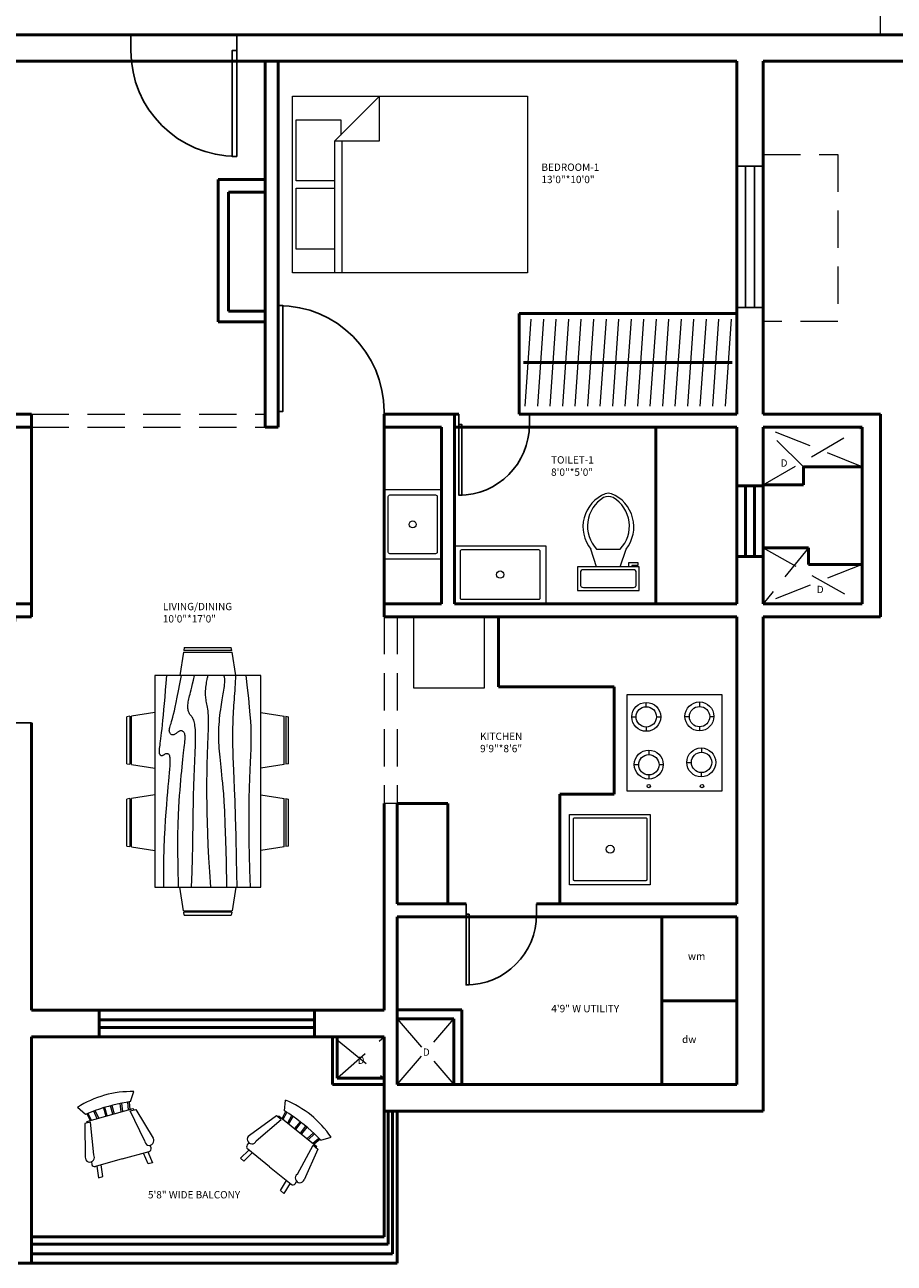
# Model space of a CAD drawing. Units: inches. Extents: x 291 to 2631, y 456 to 2623.
# Tile 5 of 22: x 1167 to 1463, y 513 to 934. Entities that reach past the tile are written whole.
import ezdxf

# ---------------------------------------------------------------- set-up
doc = ezdxf.new("R2010")
doc.units = ezdxf.units.IN
doc.linetypes.add('DASHED', pattern=[19.05, 12.7, -6.35])
for name, color, linetype, lineweight in [('A-ANNO-TEXT', 3, 'Continuous', 25), ('A-AREA-IDEN', 7, 'Continuous', 25), ('A-DOOR', 3, 'Continuous', 25), ('A-EQPM', 8, 'Continuous', 18), ('A-FLOR-FIXT', 9, 'Continuous', 18), ('A-FLOR-OVHD', 1, 'DASHED', 18), ('A-FURN', 8, 'Continuous', 18), ('A-GLAZ', 4, 'Continuous', 25), ('A-WALL', 7, 'Continuous', 50)]:
    doc.layers.add(name, color=color, linetype=linetype, lineweight=lineweight)
doc.styles.get("Standard").update_dxf_attribs({"font": 'arial.ttf'})

# ---------------------------------------------------------------- blocks, each defined once
blk = doc.blocks.new('*U2')
for p, q in [((0, 0), (0, -6)), ((40, 0), (40, -6))]:
    blk.add_line(p, q)
blk.add_lwpolyline([(0, 0), (0, 40), (1.75, 40), (1.75, 0)], close=True)
blk.add_arc((0, 0), 40, 0, 90)
blk = doc.blocks.new('Toilet - top')
for p, q in [((9.5, -6), (9.5, -2)), ((-8, -8.5), (-8, -8)), ((-7, -8), (-7, -9.5)), ((-4, -8), (-6, -14)), ((4, -8), (6, -14)), ((-10, -8.5), (-8, -8.5)), ((-10, -9.5), (-10, -8.5)), ((-7, -9.5), (-10, -9.5)), ((4, -14), (-4, -14))]:
    blk.add_line(p, q)
blk.add_lwpolyline([(10.5, -8), (10.5, 0), (-10.5, 0), (-10.5, -8)], close=True)
for points in [[(-9.5, -2), (-9.5, -6)], [(8.5, -1), (-8.5, -1)], [(-8.5, -7), (8.5, -7)]]:
    blk.add_lwpolyline(points)
for centre, radius, start, end in [((-8.62, -1.88), 0.884, 81.8699, 188.1301), ((8.62, -1.88), 0.884, 351.8699, 98.1301), ((-8.62, -6.12), 0.884, 171.8699, 278.1301), ((8.62, -6.12), 0.884, 261.8699, 8.1301), ((3.52, -21.58), 12.17, 141.4691, 247.9714), ((4.2, -21.82), 11.33, 136.3677, 238.9468), ((-3.52, -21.58), 12.17, 292.0284, 38.5307), ((-4.2, -21.82), 11.33, 301.053, 43.6321), ((0, -27.88), 4, 245.7318, 294.2682), ((0, -29), 4, 254.8605, 285.1395)]:
    blk.add_arc(centre, radius, start, end)
blk = doc.blocks.new('Dining Set - 36 x 72 in.')
for p, q in [((-22.2343, 26.00059), (-23.4847, 17.99762)), ((-22.2304, 26), (-5.7608, 26)), ((-22, 27.5), (-22.1562, 26.50042)), ((-5.8416, 26.5), (-22.1534, 26.5)), ((-22, 27.5), (-6, 27.5)), ((-5.8437, 26.49966), (-6, 27.5)), ((-4.5152, 17.99762), (-5.7655, 25.99926)), ((5.7657, 26.00059), (4.5153, 17.99762)), ((5.7696, 26), (22.2392, 26)), ((6, 27.5), (5.8438, 26.50042)), ((22.1584, 26.5), (5.8466, 26.5)), ((6, 27.5), (22, 27.5)), ((22.1563, 26.49966), (22, 27.5)), ((23.4848, 17.99762), (22.2345, 25.99926)), ((36, 18), (-36, 18)), ((-36, 18), (-36, -18)), ((36, -18), (36, 18)), ((-44.0006, 8.23428), (-35.9976, 9.48474)), ((44.0006, 8.23428), (35.9976, 9.48474)), ((-45.5, 8), (-44.5004, 8.15617)), ((-45.5, 8), (-45.5, -8)), ((-44.5, -8.15843), (-44.5, 8.15338)), ((-44, 8.23041), (-44, -8.23915)), ((44, 8.23041), (44, -8.23915)), ((44.5, -8.15843), (44.5, 8.15338)), ((45.5, 8), (44.5005, 8.15617)), ((45.5, 8), (45.5, -8)), ((-44.4997, -8.15631), (-45.5, -8)), ((-35.9976, -9.48476), (-43.9993, -8.2345)), ((35.9976, -9.48476), (43.9993, -8.2345)), ((44.4997, -8.15631), (45.5, -8)), ((-36, -18), (36, -18)), ((-22.2343, -26.0006), (-23.4847, -17.99762)), ((-4.5152, -17.99762), (-5.7655, -25.99928)), ((5.7657, -26.0006), (4.5153, -17.99762)), ((23.4848, -17.99762), (22.2345, -25.99928)), ((-22.2304, -26), (-5.7608, -26)), ((-22, -27.5), (-22.1562, -26.50044)), ((-5.8416, -26.5), (-22.1534, -26.5)), ((-22, -27.5), (-6, -27.5)), ((-5.8437, -26.49967), (-6, -27.5)), ((5.7696, -26), (22.2392, -26)), ((6, -27.5), (5.8438, -26.50044)), ((22.1584, -26.5), (5.8466, -26.5)), ((6, -27.5), (22, -27.5)), ((22.1563, -26.49967), (22, -27.5))]:
    blk.add_line(p, q)
for points in [[(-36, 15), (-31.1772, 14.97754), (-26.8079, 14.91406), (-22.8538, 14.81543), (-19.276, 14.6875), (-16.0362, 14.53613), (-13.0957, 14.36718), (-10.4159, 14.18652), (-7.9583, 14), (-5.6904, 13.81315), (-3.6035, 13.63021), (-1.6954, 13.45508), (0.0365, 13.29166), (1.5945, 13.14388), (2.9811, 13.01562), (4.1988, 12.9108), (5.25, 12.83333), (6.1393, 12.78613), (6.8802, 12.76823), (7.4883, 12.77767), (7.9792, 12.8125), (8.3685, 12.87077), (8.6719, 12.95052), (8.9049, 13.0498), (9.0833, 13.16666), (9.2205, 13.29899), (9.3216, 13.44401), (9.3895, 13.59879), (9.4271, 13.76041), (9.4373, 13.92594), (9.4232, 14.09245), (9.3875, 14.257), (9.3333, 14.41666), (9.2638, 14.56917), (9.1836, 14.71484), (9.0975, 14.85465), (9.0104, 14.98958), (8.9272, 15.1206), (8.8529, 15.2487), (8.7922, 15.37483), (8.75, 15.5), (8.7305, 15.62467), (8.7344, 15.74739), (8.7617, 15.86621), (8.8125, 15.97916), (8.8867, 16.08431), (8.9844, 16.17968), (9.1055, 16.26334), (9.25, 16.33333), (9.4189, 16.38802), (9.6172, 16.42708), (9.8506, 16.45052), (10.125, 16.45833), (10.4463, 16.45052), (10.8203, 16.42708), (11.2529, 16.38802), (11.75, 16.33333), (12.3184, 16.26318), (12.9694, 16.17838), (13.7151, 16.07991), (14.5677, 15.96875), (15.5395, 15.84586), (16.6426, 15.71224), (17.8893, 15.56884), (19.2917, 15.41666), (20.859, 15.25667), (22.5879, 15.08984), (24.4721, 14.91715), (26.5052, 14.73958), (28.6809, 14.5581), (30.9929, 14.3737), (33.4347, 14.18733), (36, 14)], [(-36, 10), (-28.9766, 10.14274), (-23.1725, 10.20442), (-18.4241, 10.19775), (-14.5677, 10.13541), (-11.4399, 10.03011), (-8.877, 9.89453), (-6.7154, 9.74137), (-4.7917, 9.58333), (-2.9698, 9.43082), (-1.2246, 9.28515), (0.4415, 9.14534), (2.026, 9.01041), (3.5266, 8.87939), (4.9408, 8.7513), (6.266, 8.62516), (7.5, 8.5), (8.6411, 8.37549), (9.6914, 8.2539), (10.6538, 8.13818), (11.5312, 8.03125), (12.3267, 7.93603), (13.043, 7.85547), (13.6831, 7.79248), (14.25, 7.75), (14.7471, 7.7303), (15.1797, 7.73307), (15.5537, 7.75732), (15.875, 7.80208), (16.1494, 7.86637), (16.3828, 7.94922), (16.5811, 8.04964), (16.75, 8.16666), (16.8944, 8.29915), (17.0143, 8.44531), (17.1089, 8.60319), (17.1771, 8.77083), (17.218, 8.94629), (17.2305, 9.1276), (17.2137, 9.31282), (17.1667, 9.5), (17.0895, 9.6875), (16.987, 9.875), (16.8649, 10.0625), (16.7292, 10.25), (16.5856, 10.4375), (16.4401, 10.625), (16.2985, 10.8125), (16.1667, 11), (16.05, 11.18733), (15.9518, 11.3737), (15.8752, 11.5581), (15.8229, 11.73958), (15.798, 11.91715), (15.8034, 12.08984), (15.842, 12.25667), (15.9167, 12.41666), (16.0295, 12.56836), (16.1784, 12.70833), (16.3605, 12.83268), (16.5729, 12.9375), (16.8127, 13.01888), (17.0768, 13.07291), (17.3625, 13.0957), (17.6667, 13.08333), (17.9894, 13.03312), (18.3418, 12.94726), (18.7382, 12.82918), (19.1927, 12.68229), (19.7195, 12.51001), (20.3327, 12.31575), (21.0465, 12.10294), (21.875, 11.875), (22.8357, 11.63354), (23.959, 11.37304), (25.2786, 11.08618), (26.8282, 10.76562), (28.6414, 10.40405), (30.752, 9.99414), (33.1936, 9.52856), (36, 9)], [(-36, 5.5), (-30.7157, 5.3348), (-26.069, 5.20963), (-21.9946, 5.11767), (-18.4271, 5.05208), (-15.3009, 5.00602), (-12.5508, 4.97265), (-10.1112, 4.94515), (-7.9167, 4.91666), (-5.909, 4.88167), (-4.0586, 4.83984), (-2.3429, 4.79215), (-0.7396, 4.73958), (0.7739, 4.6831), (2.22, 4.6237), (3.6213, 4.56233), (5, 4.5), (6.373, 4.43782), (7.7344, 4.3776), (9.0723, 4.32129), (10.375, 4.27083), (11.6309, 4.22819), (12.8281, 4.19531), (13.9551, 4.17415), (15, 4.16666), (15.954, 4.17448), (16.819, 4.19791), (17.6001, 4.23698), (18.3021, 4.29166), (18.9299, 4.36198), (19.4883, 4.44791), (19.9823, 4.54948), (20.4167, 4.66666), (20.7969, 4.79899), (21.1302, 4.94401), (21.4245, 5.09879), (21.6875, 5.26041), (21.9271, 5.42594), (22.1511, 5.59245), (22.3672, 5.757), (22.5834, 5.91666), (22.8065, 6.06868), (23.0404, 6.21093), (23.2879, 6.34147), (23.5521, 6.45833), (23.8358, 6.55957), (24.142, 6.64323), (24.4735, 6.70735), (24.8334, 6.75), (25.2235, 6.76969), (25.642, 6.76692), (26.0858, 6.74267), (26.5521, 6.69791), (27.0379, 6.63362), (27.5404, 6.55078), (28.0565, 6.45036), (28.5834, 6.33333), (29.1242, 6.19987), (29.7071, 6.04687), (30.3661, 5.87044), (31.1354, 5.66666), (32.0493, 5.43164), (33.142, 5.16146), (34.4475, 4.85221), (36, 4.5)], [(-36, -1), (-30.7915, -0.6591), (-26.0195, -0.38216), (-21.6519, -0.16284), (-17.6563, 0.00521), (-14.0005, 0.12833), (-10.6523, 0.21289), (-7.5796, 0.26522), (-4.75, 0.29166), (-2.134, 0.29793), (0.2878, 0.28711), (2.5317, 0.26163), (4.6146, 0.22396), (6.5529, 0.17651), (8.3633, 0.12174), (10.0623, 0.06209), (11.6667, 0), (13.1899, -0.06201), (14.6341, -0.1211), (15.9982, -0.17432), (17.2813, -0.21875), (18.4823, -0.25147), (19.6003, -0.26953), (20.6343, -0.27002), (21.5834, -0.25), (22.4481, -0.20768), (23.2357, -0.14584), (23.9549, -0.06836), (24.6146, 0.02083), (25.2235, 0.11784), (25.7904, 0.21875), (26.3241, 0.31966), (26.8334, 0.41666), (27.3265, 0.50618), (27.8099, 0.58593), (28.2894, 0.65397), (28.7709, 0.70833), (29.2601, 0.74707), (29.763, 0.76823), (30.2855, 0.76985), (30.8334, 0.75), (31.4088, 0.70784), (31.9994, 0.64713), (32.589, 0.57275), (33.1615, 0.48958), (33.7008, 0.4025), (34.1908, 0.3164), (34.6153, 0.23616), (34.9584, 0.16666), (35.2099, 0.11165), (35.3848, 0.07031), (35.504, 0.04069), (35.5886, 0.02083), (35.6594, 0.00879), (35.7377, 0.0026), (35.8442, 0.00032), (36, 0)], [(-36, -6.5), (-27.1843, -6.31267), (-20.084, -6.1263), (-14.469, -5.9419), (-10.1094, -5.76042), (-6.7752, -5.58285), (-4.2363, -5.41016), (-2.2629, -5.24333), (-0.625, -5.08334), (0.8708, -4.93099), (2.2715, -4.78646), (3.5872, -4.64974), (4.8281, -4.52084), (6.0046, -4.39974), (7.127, -4.28646), (8.2053, -4.18099), (9.25, -4.08334), (10.2705, -3.99382), (11.2734, -3.91407), (12.2647, -3.84603), (13.25, -3.79167), (14.2354, -3.75293), (15.2266, -3.73177), (16.2295, -3.73015), (17.25, -3.75), (18.2912, -3.79248), (19.3451, -3.85547), (20.4009, -3.93604), (21.4479, -4.03125), (22.4754, -4.13819), (23.4727, -4.25391), (24.4289, -4.37549), (25.3334, -4.5), (26.1785, -4.62492), (26.9694, -4.74935), (27.7145, -4.87281), (28.4219, -4.99479), (29.1, -5.11483), (29.7572, -5.23242), (30.4016, -5.34709), (31.0417, -5.45834), (31.6837, -5.56437), (32.3262, -5.65821), (32.9658, -5.73153), (33.599, -5.77604), (34.2224, -5.78345), (34.8327, -5.74545), (35.4264, -5.65373), (36, -5.5)], [(-36, -10), (-26.4022, -9.81299), (-18.4675, -9.62891), (-11.9839, -9.45069), (-6.7396, -9.28125), (-2.5226, -9.12354), (0.8789, -8.98047), (3.6769, -8.85498), (6.0833, -8.75), (8.2767, -8.66765), (10.3021, -8.60677), (12.1712, -8.56543), (13.8958, -8.54167), (15.4876, -8.53353), (16.9583, -8.53907), (18.3197, -8.55632), (19.5834, -8.58334), (20.7616, -8.61841), (21.8685, -8.66081), (22.9188, -8.71004), (23.9271, -8.76563), (24.9081, -8.82707), (25.8763, -8.89388), (26.8465, -8.96558), (27.8334, -9.04167), (28.8474, -9.12118), (29.8828, -9.20117), (30.93, -9.27824), (31.9792, -9.34896), (33.0205, -9.40991), (34.0443, -9.45768), (35.0407, -9.48885), (36, -9.5)], [(-36, -14.5), (-30.0881, -14.33513), (-25.0332, -14.21224), (-20.7312, -14.12647), (-17.0781, -14.07292), (-13.97, -14.04671), (-11.3027, -14.04297), (-8.9724, -14.05681), (-6.875, -14.08334), (-4.9224, -14.11833), (-3.0905, -14.16016), (-1.3709, -14.20785), (0.2448, -14.26042), (1.7647, -14.3169), (3.1973, -14.3763), (4.5507, -14.43767), (5.8333, -14.5), (7.0554, -14.5621), (8.235, -14.62175), (9.3922, -14.67652), (10.5469, -14.72396), (11.7192, -14.76164), (12.929, -14.78711), (14.1965, -14.79794), (15.5417, -14.79167), (16.9933, -14.76424), (18.6152, -14.70508), (20.4804, -14.60197), (22.6615, -14.44271), (25.2312, -14.21509), (28.2624, -13.9069), (31.8277, -13.50594), (36, -13)]]:
    blk.add_lwpolyline(points)
blk = doc.blocks.new('Chair - Rocking')
for p, q in [((-8, -4.5), (-10, -1.5)), ((-4.5, -7), (-4.96674, -4.19951)), ((-4, -7), (-4.40532, -4.16272)), ((-1.5, -4.05012), (-1.5, -7)), ((-1, -7), (-1, -4.05012)), ((1, -7), (1, -4.04655)), ((1.5, -4.05012), (1.5, -7)), ((4, -7), (4.40187, -4.18694)), ((4.5, -7), (4.96761, -4.19437)), ((8, -4.5), (10, -1.5)), ((-9, -7.5), (-12, -18.49999)), ((-7, -7.5), (-9, -7.5)), ((-9, -18.49999), (-7, -7.5)), ((-8.23428, -6.99939), (-8.3093, -7.47958)), ((-8.23041, -7), (8.23915, -7)), ((-7.5, -4.5), (-7, -7)), ((-6.5, -7), (-7.02225, -4.43)), ((6.5, -7), (7, -4.4057)), ((7.5, -4.5), (7, -7)), ((7, -7.5), (9, -7.5)), ((9, -18.49999), (7, -7.5)), ((8.31071, -7.48854), (8.23449, -7.00073)), ((9, -7.5), (12, -18.49999)), ((-10.36644, -20.64523), (-10.5, -21.49999)), ((10.5, -21.49999), (10.3575, -20.58798)), ((-9, -22.49999), (-9.5, -26.49999)), ((0, -22.49999), (-9.5, -22.49999)), ((-8, -26.49999), (-7.5, -22.49999)), ((0, -22.49999), (9.5, -22.49999)), ((8, -26.49999), (7.5, -22.49999)), ((9, -22.49999), (9.5, -26.49999)), ((-9.5, -26.49999), (-8, -26.49999)), ((9.5, -26.49999), (8, -26.49999))]:
    blk.add_line(p, q)
for centre, radius, start, end in [((0, -34.08333), 34.08333, 72.93847, 107.0615), ((0, -68.25004), 64.25, 93.92211, 97.15267), ((0, -68.25004), 64.25, 82.84733, 93.92211), ((-10.5, -18.99999), 1.58114, 161.5651, 18.43495), ((10.5, -18.99999), 1.58114, 161.5651, 18.43495), ((-9.5, -21.49999), 1, 180, 270), ((9.5, -21.49999), 1, 270, 0)]:
    blk.add_arc(centre, radius, start, end)
blk = doc.blocks.new('Bed - Queen')
for p, q in [((0, -80.00003), (0, 0)), ((0, 0), (59.99999, 0)), ((59.99999, 0), (59.99999, -80.00003)), ((7.99999, -1.2), (28.79998, -1.2)), ((7.99999, -14.4), (7.99999, -1.2)), ((28.79998, -1.2), (28.79998, -14.4)), ((31.19999, -1.2), (51.99999, -1.2)), ((31.19999, -14.4), (31.19999, -1.2)), ((51.99999, -1.2), (51.99999, -16.4)), ((0, -14.4), (44.8, -14.4)), ((44.8, -16.8), (0, -16.8)), ((59.99999, -29.6), (44.8, -14.4)), ((44.8, -14.4), (44.8, -29.6)), ((51.99999, -16.4), (46.79936, -16.4)), ((44.8, -29.6), (59.99999, -29.6)), ((59.99999, -80.00003), (0, -80.00003))]:
    blk.add_line(p, q)
blk = doc.blocks.new('WIN-1200')
for p, q in [((0, 0), (0, 48)), ((0, 48), (9, 48)), ((3, 0), (3, 48)), ((6, 48), (6, 0)), ((9, 48), (9, 0)), ((9, 0), (0, 0))]:
    blk.add_line(p, q)
blk = doc.blocks.new('COOKTOP-B')
for p, q in [((6.54, 28.68), (6.54, 30.14)), ((24.62, 30.31), (24.62, 28.76)), ((19.7, 25.39), (21.21, 25.39)), ((28.13, 25.39), (29.54, 25.39)), ((1.62, 25.22), (3.08, 25.22)), ((6.54, 21.76), (6.54, 20.3)), ((10, 25.22), (11.46, 25.22)), ((24.62, 21.83), (24.62, 20.47)), ((7.38, 13.92), (7.38, 12.38)), ((25.35, 14.65), (25.34, 13.21)), ((2.46, 9), (3.95, 9)), ((10.87, 9), (12.3, 9)), ((20.32, 9.73), (21.89, 9.73)), ((7.38, 5.46), (7.38, 4.08)), ((25.26, 6.28), (25.24, 4.81))]:
    blk.add_line(p, q)
blk.add_lwpolyline([(0, 32.79), (32.25, 32.79), (32.25, 0), (0, 0)], close=True)
for centre, radius in [((6.54, 25.22), 4.92), ((24.62, 25.39), 4.92), ((6.54, 25.22), 3.46), ((24.67, 25.29), 3.46), ((7.38, 9), 4.92), ((25.24, 9.73), 4.92), ((25.35, 9.74), 3.46), ((7.41, 8.92), 3.46), ((7.38, 1.69), 0.572), ((25.5, 1.69), 0.572)]:
    blk.add_circle(centre, radius)

msp = doc.modelspace()

# ---------------------------------------------------------------- linework, layer by layer
at = {"layer": 'A-FLOR-OVHD'}
for p, q in [((1458.34, 1111.65), (1458.34, 930.98)), ((1418.5, 890.21), (1443.93, 890.21)), ((1443.93, 890.21), (1443.93, 833.45)), ((1443.93, 833.45), (1418.5, 833.45)), ((1169.5, 801.98), (1249, 801.98)), ((1169.5, 797.48), (1249, 797.48)), ((1452.18, 784.08), (1418.5, 797.48)), ((1418.5, 777.9), (1452.18, 797.48)), ((1432.19, 784.08), (1418.5, 797.48)), ((1418.5, 756.5), (1452.18, 737.48)), ((1433.89, 756.5), (1418.5, 737.48)), ((1452.18, 750.84), (1418.5, 737.48)), ((1289.5, 732.98), (1289.5, 669.54)), ((1294, 732.98), (1294, 669.54)), ((1294, 669.54), (1289.5, 669.54)), ((1294, 596.39), (1313.26, 573.98)), ((1294, 573.98), (1313.26, 596.39)), ((1273.6, 590.24), (1273.6, 589.22)), ((1273.6, 576.12), (1289.5, 590.24)), ((1273.6, 589.22), (1289.5, 576.12))]:
    msp.add_line(p, q, dxfattribs=at)
at = {"layer": 'A-FURN'}
for p, q in [((1337.54, 804.7), (1339.61, 834.23)), ((1341.8, 804.7), (1343.86, 834.23)), ((1346.05, 804.7), (1348.12, 834.23)), ((1350.31, 804.7), (1352.37, 834.23)), ((1354.56, 804.7), (1356.63, 834.23)), ((1358.82, 804.7), (1360.88, 834.23)), ((1363.07, 804.7), (1365.14, 834.23)), ((1367.33, 804.7), (1369.4, 834.23)), ((1371.59, 804.7), (1373.65, 834.23)), ((1375.84, 804.7), (1377.91, 834.23)), ((1380.1, 804.7), (1382.16, 834.23)), ((1384.35, 804.7), (1386.42, 834.23)), ((1388.61, 804.7), (1390.68, 834.23)), ((1392.86, 804.7), (1394.93, 834.23)), ((1397.12, 804.7), (1399.19, 834.23)), ((1401.38, 804.7), (1403.44, 834.23)), ((1405.63, 804.7), (1407.7, 834.23))]:
    msp.add_line(p, q, dxfattribs=at)
for points in [[(1289.5, 776.29), (1309, 776.29), (1309, 752.63), (1289.5, 752.63)], [(1313.5, 737.48), (1344.66, 737.48), (1344.66, 757.06), (1313.5, 757.06)], [(1299.65, 732.98), (1323.58, 732.98), (1323.58, 708.81), (1299.65, 708.81)], [(1352.65, 665.8), (1380.09, 665.8), (1380.09, 641.9), (1352.65, 641.9)]]:
    msp.add_lwpolyline(points, close=True, dxfattribs=at)
for points in [[(1291.46, 774.47), (1307.06, 774.47, -0.414214), (1307.56, 773.97), (1307.56, 755, -0.414214), (1307.06, 754.5), (1291.46, 754.5, -0.414214), (1290.96, 755), (1290.96, 773.97, -0.414214)], [(1315.87, 739), (1342.16, 739, 0.414214), (1342.66, 739.5), (1342.66, 755.27, 0.414214), (1342.16, 755.77), (1315.87, 755.77, 0.414214), (1315.37, 755.27), (1315.37, 739.5, 0.414214)], [(1354.29, 664.69), (1378.59, 664.69, -0.414214), (1378.89, 664.39), (1378.89, 643.61, -0.414214), (1378.59, 643.31), (1354.29, 643.31, -0.414214), (1353.99, 643.61), (1353.99, 664.39, -0.414214)]]:
    msp.add_lwpolyline(points, format="xyb", close=True, dxfattribs=at)
for centre, radius in [((1299.26, 764.48), 1.16), ((1329.01, 747.38), 1.24), ((1366.44, 654), 1.36)]:
    msp.add_circle(centre, radius, dxfattribs=at)
at = {"layer": 'A-WALL'}
for p, q in [((1989.87, 930.98), (1024, 930.98)), ((1409.5, 921.98), (1033, 921.98)), ((1249, 921.98), (1249, 797.48)), ((1253.5, 921.98), (1253.5, 797.48)), ((1409.5, 921.98), (1409.5, 801.98)), ((1595.37, 921.98), (1418.5, 921.98)), ((1418.5, 921.98), (1418.5, 801.98)), ((1249, 881.72), (1233.03, 881.72)), ((1233.03, 881.72), (1233.03, 833.39)), ((1249, 877.47), (1236.59, 877.47)), ((1236.59, 877.47), (1236.59, 836.95)), ((1236.59, 836.95), (1249, 836.95)), ((1335.52, 801.98), (1335.52, 836.12)), ((1335.52, 836.12), (1409.5, 836.12)), ((1233.03, 833.39), (1249, 833.39)), ((1336.9, 819.47), (1407.94, 819.47)), ((1169.5, 801.98), (1033, 801.98)), ((1169.5, 737.48), (1169.5, 801.98)), ((1289.5, 737.48), (1289.5, 801.98)), ((1314.97, 801.98), (1289.5, 801.98)), ((1313.5, 801.98), (1313.5, 737.48)), ((1409.5, 801.98), (1335.52, 801.98)), ((1418.5, 801.98), (1458.38, 801.98)), ((1458.38, 801.98), (1458.38, 732.98)), ((1169.5, 797.48), (1145.5, 797.48)), ((1253.5, 797.48), (1249, 797.48)), ((1309, 797.48), (1289.5, 797.48)), ((1309, 797.48), (1309, 737.48)), ((1409.5, 797.48), (1313.5, 797.48)), ((1381.97, 797.48), (1381.97, 737.48)), ((1409.5, 797.48), (1409.5, 737.48)), ((1418.5, 797.48), (1452.18, 797.48)), ((1418.5, 797.48), (1418.5, 737.48)), ((1452.18, 797.48), (1452.18, 737.48)), ((1432.19, 777.9), (1432.19, 784.08)), ((1432.19, 784.08), (1452.18, 784.08)), ((1418.5, 777.55), (1409.5, 777.55)), ((1409.5, 777.55), (1409.5, 753.55)), ((1412.5, 777.55), (1412.5, 753.55)), ((1415.5, 753.55), (1415.5, 777.55)), ((1418.5, 777.9), (1432.19, 777.9)), ((1418.5, 753.55), (1418.5, 777.55)), ((1418.5, 756.5), (1433.89, 756.5)), ((1433.89, 756.5), (1433.89, 750.84)), ((1409.5, 753.55), (1418.5, 753.55)), ((1433.89, 750.84), (1452.18, 750.84)), ((1169.5, 737.48), (1145.5, 737.48)), ((1169.5, 737.48), (1169.5, 732.98)), ((1289.5, 737.48), (1289.5, 732.98)), ((1309, 737.48), (1289.5, 737.48)), ((1409.5, 737.48), (1313.5, 737.48)), ((1452.18, 737.48), (1418.5, 737.48)), ((1169.5, 732.98), (1105.76, 732.98)), ((1409.5, 732.98), (1289.5, 732.98)), ((1328.43, 709.22), (1328.43, 732.98)), ((1409.5, 732.98), (1409.5, 635.48)), ((1458.38, 732.98), (1418.5, 732.98)), ((1418.5, 732.98), (1418.5, 564.98)), ((1367.84, 709.22), (1328.43, 709.22)), ((1367.84, 672.71), (1367.84, 709.22)), ((1169.5, 696.98), (1169.5, 599.24)), ((1349.26, 635.48), (1349.26, 672.71)), ((1349.26, 672.71), (1367.84, 672.71)), ((1289.5, 669.54), (1289.5, 599.24)), ((1311.16, 669.54), (1294, 669.54)), ((1294, 669.54), (1294, 635.48)), ((1311.16, 635.48), (1311.16, 669.54)), ((1317.41, 635.48), (1294, 635.48)), ((1409.5, 635.48), (1341.41, 635.48)), ((1409.5, 630.98), (1294, 630.98)), ((1294, 630.98), (1294, 573.98)), ((1383.99, 630.98), (1383.99, 573.98)), ((1409.5, 630.98), (1409.5, 573.98)), ((1383.99, 602.48), (1409.5, 602.48)), ((1169.5, 599.24), (1289.5, 599.24)), ((1192.62, 599.24), (1192.62, 590.24)), ((1265.84, 599.24), (1265.84, 590.24)), ((1294, 599.4), (1315.99, 599.4)), ((1315.99, 599.4), (1315.99, 573.98)), ((1192.62, 595.97), (1265.84, 595.97)), ((1294, 596.39), (1313.26, 596.39)), ((1313.26, 596.39), (1313.26, 573.98)), ((1169.5, 590.24), (1289.5, 590.24)), ((1169.5, 590.24), (1169.5, 564.98)), ((1192.62, 593.4), (1265.84, 593.4)), ((1272, 573.98), (1272, 590.24)), ((1273.6, 590.24), (1273.6, 576.12)), ((1289.5, 590.24), (1289.5, 522.24)), ((1289.5, 573.98), (1272, 573.98)), ((1273.6, 576.12), (1289.5, 576.12)), ((1409.5, 573.98), (1294, 573.98)), ((1169.5, 564.98), (1169.5, 513.24)), ((1418.5, 564.98), (1289.5, 564.98)), ((1290.92, 519.67), (1290.92, 564.98)), ((1292.35, 564.98), (1292.35, 516.49)), ((1294, 564.98), (1294, 513.24)), ((1169.5, 522.24), (1289.5, 522.24)), ((1169.54, 519.67), (1290.92, 519.67)), ((1292.35, 516.49), (1169.5, 516.49)), ((1165, 513.24), (1169.5, 513.24)), ((1169.5, 513.24), (1289.5, 513.24)), ((1294, 513.24), (1289.5, 513.24))]:
    msp.add_line(p, q, dxfattribs=at)

# ---------------------------------------------------------------- block references
at = {"layer": 'A-DOOR'}
for p, xscale, yscale, zscale, rotation in [((1239.36, 925.58), 0.9, 0.9, 0.9, 180), ((1314.97, 798.38), -0.6, 0.6, 0.6, 180), ((1164.1, 732.98), -0.9, 0.9, 0.9, 90), ((1317.41, 631.88), -0.6, 0.6, 0.6, 180)]:
    msp.add_blockref('*U2', p, dxfattribs=dict(at, xscale=xscale, yscale=yscale, zscale=zscale, rotation=rotation))
at = {"layer": 'A-DOOR', "xscale": 0.9, "yscale": 0.9, "zscale": 0.9}
msp.add_blockref('*U2', (1253.5, 802.88), dxfattribs=at)
at = {"layer": 'A-EQPM'}
msp.add_blockref('COOKTOP-B', (1372.19, 673.8), dxfattribs=at)
at = {"layer": 'A-FLOR-FIXT', "rotation": 180}
msp.add_blockref('Toilet - top', (1365.84, 742.03), dxfattribs=at)
at = {"layer": 'A-FURN'}
for name, p, rotation in [('Bed - Queen', (1258.35, 850.03), 90), ('Dining Set - 36 x 72 in.', (1229.54, 677.06), 90), ('Chair - Rocking', (1194.37, 570.35), 15.67595765379025), ('Chair - Rocking', (1264.65, 563.57), 321.0741999402937)]:
    msp.add_blockref(name, p, dxfattribs=dict(at, rotation=rotation))
at = {"layer": 'A-GLAZ'}
msp.add_blockref('WIN-1200', (1409.5, 838.26), dxfattribs=at)

# ---------------------------------------------------------------- texts
at = {"layer": 'A-ANNO-TEXT', "char_height": 2.5, "attachment_point": 1}
for s, width, insert in [('D', 4.3342, (1424.43, 786.58)), ('D', 3.7027, (1436.72, 743.58)), ('wm', 15.5024, (1392.91, 618.89)), ('dw', 11.393, (1390.91, 590.61)), ('D', 2.0474, (1302.7, 586.26)), ('D', 2.105, (1280.51, 583.53))]:
    msp.add_mtext_dynamic_manual_height_columns(s, width=width, gutter_width=12.5, heights=[0], dxfattribs=dict(at, insert=insert))
at = {"layer": 'A-AREA-IDEN', "char_height": 2.5, "attachment_point": 1}
for s, width, insert in [('BEDROOM-1\\P13\'0"*10\'0"', 60.4042, (1343.06, 887.16)), ('TOILET-1\\P8\'0"*5\'0"', 33.7546, (1346.33, 787.64)), ('LIVING/DINING\\P10\'0"*17\'0"', 73.7754, (1214.24, 737.78)), ('KITCHEN\\P9\'9"*8\'6"', 47.0988, (1322.18, 693.66)), ('4\'9" W UTILITY', 52.2192, (1346.41, 601.08)), ('5\'8" WIDE BALCONY', 55.0782, (1209.17, 537.78))]:
    msp.add_mtext_dynamic_manual_height_columns(s, width=width, gutter_width=12.5, heights=[0], dxfattribs=dict(at, insert=insert))

doc.saveas('drawing.dxf')
